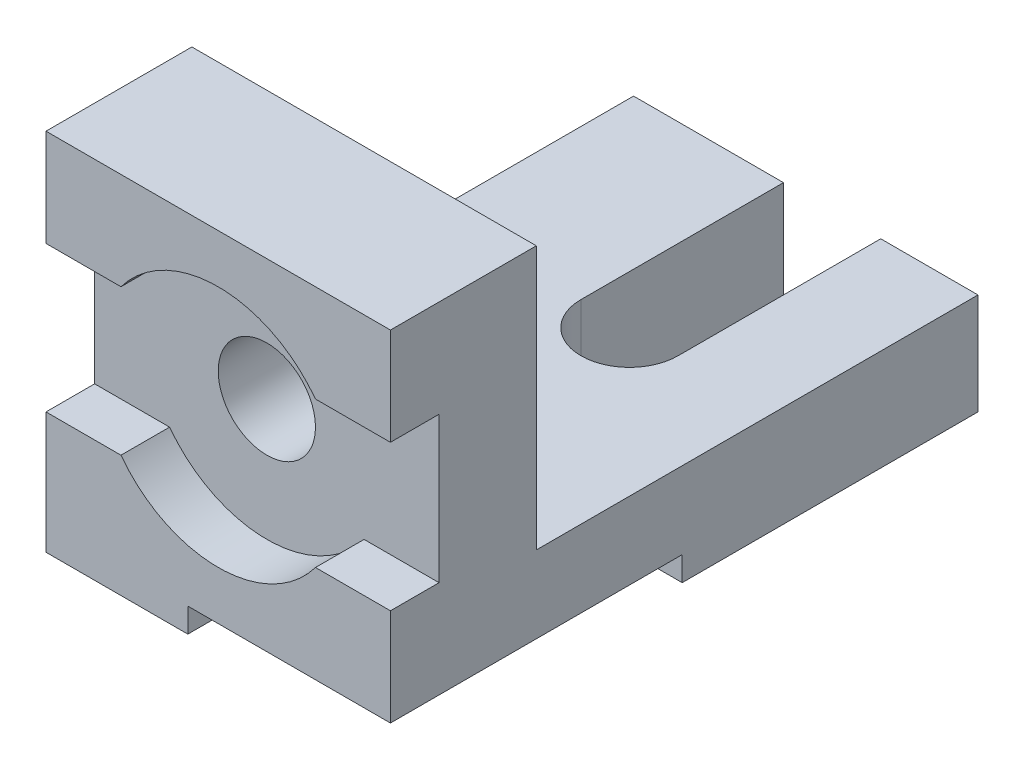
ISO-10303-21;
HEADER;
FILE_DESCRIPTION(('STEP AP214'),'2;1');
FILE_NAME('part.step','',(''),(''),'','','');
FILE_SCHEMA(('AUTOMOTIVE_DESIGN { 1 0 10303 214 1 1 1 1 }'));
ENDSEC;
DATA;
#1=APPLICATION_CONTEXT('core data for automotive mechanical design processes');
#2=APPLICATION_PROTOCOL_DEFINITION('international standard','automotive_design',2000,#1);
#3=PRODUCT_CONTEXT('',#1,'mechanical');
#4=PRODUCT('Part','Part','',(#3));
#5=PRODUCT_RELATED_PRODUCT_CATEGORY('part','',(#4));
#6=PRODUCT_DEFINITION_FORMATION('','',#4);
#7=PRODUCT_DEFINITION_CONTEXT('part definition',#1,'design');
#8=PRODUCT_DEFINITION('design','',#6,#7);
#9=PRODUCT_DEFINITION_SHAPE('','',#8);
#10=(LENGTH_UNIT() NAMED_UNIT(*) SI_UNIT(.MILLI.,.METRE.));
#11=(NAMED_UNIT(*) PLANE_ANGLE_UNIT() SI_UNIT($,.RADIAN.));
#12=(NAMED_UNIT(*) SI_UNIT($,.STERADIAN.) SOLID_ANGLE_UNIT());
#13=UNCERTAINTY_MEASURE_WITH_UNIT(LENGTH_MEASURE(1.E-05),#10,'distance_accuracy_value','');
#14=(GEOMETRIC_REPRESENTATION_CONTEXT(3) GLOBAL_UNCERTAINTY_ASSIGNED_CONTEXT((#13)) GLOBAL_UNIT_ASSIGNED_CONTEXT((#10,
#11,#12)) REPRESENTATION_CONTEXT('',''));
#15=CARTESIAN_POINT('',(0.,0.,0.));
#16=DIRECTION('',(0.,0.,1.));
#17=DIRECTION('',(1.,0.,0.));
#18=AXIS2_PLACEMENT_3D('',#15,#16,#17);
#19=CARTESIAN_POINT('',(42.5,0.,95.));
#20=DIRECTION('',(0.,0.,-1.));
#21=DIRECTION('',(-1.,0.,0.));
#22=AXIS2_PLACEMENT_3D('',#19,#20,#21);
#23=PLANE('',#22);
#24=DIRECTION('',(1.,0.,0.));
#25=VECTOR('',#24,1.);
#26=CARTESIAN_POINT('',(0.,30.,95.));
#27=LINE('',#26,#25);
#28=CARTESIAN_POINT('',(-42.5,30.,95.));
#29=VERTEX_POINT('',#28);
#30=CARTESIAN_POINT('',(-24.,30.,95.));
#31=VERTEX_POINT('',#30);
#32=EDGE_CURVE('E229',#29,#31,#27,.T.);
#33=ORIENTED_EDGE('',*,*,#32,.F.);
#34=DIRECTION('',(0.,-1.,0.));
#35=VECTOR('',#34,1.);
#36=CARTESIAN_POINT('',(-42.5,0.,95.));
#37=LINE('',#36,#35);
#38=CARTESIAN_POINT('',(-42.5,0.,95.));
#39=VERTEX_POINT('',#38);
#40=EDGE_CURVE('E314',#29,#39,#37,.T.);
#41=ORIENTED_EDGE('',*,*,#40,.T.);
#42=DIRECTION('',(-1.,0.,0.));
#43=VECTOR('',#42,1.);
#44=CARTESIAN_POINT('',(42.5,0.,95.));
#45=LINE('',#44,#43);
#46=CARTESIAN_POINT('',(-7.5,0.,95.));
#47=VERTEX_POINT('',#46);
#48=EDGE_CURVE('E323',#47,#39,#45,.T.);
#49=ORIENTED_EDGE('',*,*,#48,.F.);
#50=DIRECTION('',(0.,-1.,0.));
#51=VECTOR('',#50,1.);
#52=CARTESIAN_POINT('',(-7.5,0.,95.));
#53=LINE('',#52,#51);
#54=CARTESIAN_POINT('',(-7.5,5.99999999999996,95.));
#55=VERTEX_POINT('',#54);
#56=EDGE_CURVE('E258',#55,#47,#53,.T.);
#57=ORIENTED_EDGE('',*,*,#56,.F.);
#58=DIRECTION('',(1.,0.,0.));
#59=VECTOR('',#58,1.);
#60=CARTESIAN_POINT('',(-7.5,5.99999999999996,95.));
#61=LINE('',#60,#59);
#62=CARTESIAN_POINT('',(42.5,5.99999999999996,95.));
#63=VERTEX_POINT('',#62);
#64=EDGE_CURVE('E268',#55,#63,#61,.T.);
#65=ORIENTED_EDGE('',*,*,#64,.T.);
#66=DIRECTION('',(0.,-1.,0.));
#67=VECTOR('',#66,1.);
#68=CARTESIAN_POINT('',(42.5,0.,95.));
#69=LINE('',#68,#67);
#70=CARTESIAN_POINT('',(42.5,30.,95.));
#71=VERTEX_POINT('',#70);
#72=EDGE_CURVE('E300',#71,#63,#69,.T.);
#73=ORIENTED_EDGE('',*,*,#72,.F.);
#74=DIRECTION('',(1.,0.,0.));
#75=VECTOR('',#74,1.);
#76=CARTESIAN_POINT('',(0.,30.,95.));
#77=LINE('',#76,#75);
#78=CARTESIAN_POINT('',(24.,30.,95.));
#79=VERTEX_POINT('',#78);
#80=EDGE_CURVE('E203',#79,#71,#77,.T.);
#81=ORIENTED_EDGE('',*,*,#80,.F.);
#82=CARTESIAN_POINT('',(0.,48.,95.));
#83=DIRECTION('',(0.,0.,1.));
#84=DIRECTION('',(1.,0.,0.));
#85=AXIS2_PLACEMENT_3D('',#82,#83,#84);
#86=CIRCLE('',#85,30.);
#87=EDGE_CURVE('E226',#31,#79,#86,.T.);
#88=ORIENTED_EDGE('',*,*,#87,.F.);
#89=EDGE_LOOP('',(#33,#41,#49,#57,#65,#73,#81,#88));
#90=FACE_BOUND('',#89,.T.);
#91=ADVANCED_FACE('F39',(#90),#23,.F.);
#92=CARTESIAN_POINT('',(-42.5,0.,0.));
#93=DIRECTION('',(-1.,0.,0.));
#94=DIRECTION('',(0.,0.,1.));
#95=AXIS2_PLACEMENT_3D('',#92,#93,#94);
#96=PLANE('',#95);
#97=DIRECTION('',(0.,-1.,0.));
#98=VECTOR('',#97,1.);
#99=CARTESIAN_POINT('',(-42.5,0.,83.));
#100=LINE('',#99,#98);
#101=CARTESIAN_POINT('',(-42.5,66.,83.));
#102=VERTEX_POINT('',#101);
#103=CARTESIAN_POINT('',(-42.5,30.,83.));
#104=VERTEX_POINT('',#103);
#105=EDGE_CURVE('E206',#102,#104,#100,.T.);
#106=ORIENTED_EDGE('',*,*,#105,.F.);
#107=DIRECTION('',(0.,0.,1.));
#108=VECTOR('',#107,1.);
#109=CARTESIAN_POINT('',(-42.5,66.,83.));
#110=LINE('',#109,#108);
#111=CARTESIAN_POINT('',(-42.5,66.,95.));
#112=VERTEX_POINT('',#111);
#113=EDGE_CURVE('E241',#102,#112,#110,.T.);
#114=ORIENTED_EDGE('',*,*,#113,.T.);
#115=CARTESIAN_POINT('',(-42.5,90.,95.));
#116=VERTEX_POINT('',#115);
#117=EDGE_CURVE('E312',#116,#112,#37,.T.);
#118=ORIENTED_EDGE('',*,*,#117,.F.);
#119=DIRECTION('',(0.,0.,1.));
#120=VECTOR('',#119,1.);
#121=CARTESIAN_POINT('',(-42.5,90.,95.));
#122=LINE('',#121,#120);
#123=CARTESIAN_POINT('',(-42.5,90.,59.));
#124=VERTEX_POINT('',#123);
#125=EDGE_CURVE('E315',#124,#116,#122,.T.);
#126=ORIENTED_EDGE('',*,*,#125,.F.);
#127=DIRECTION('',(0.,1.,0.));
#128=VECTOR('',#127,1.);
#129=CARTESIAN_POINT('',(-42.5,90.,59.));
#130=LINE('',#129,#128);
#131=CARTESIAN_POINT('',(-42.5,25.,59.));
#132=VERTEX_POINT('',#131);
#133=EDGE_CURVE('E309',#132,#124,#130,.T.);
#134=ORIENTED_EDGE('',*,*,#133,.F.);
#135=DIRECTION('',(0.,0.,1.));
#136=VECTOR('',#135,1.);
#137=CARTESIAN_POINT('',(-42.5,25.,59.));
#138=LINE('',#137,#136);
#139=CARTESIAN_POINT('',(-42.5,25.,-50.));
#140=VERTEX_POINT('',#139);
#141=EDGE_CURVE('E306',#140,#132,#138,.T.);
#142=ORIENTED_EDGE('',*,*,#141,.F.);
#143=DIRECTION('',(0.,1.,0.));
#144=VECTOR('',#143,1.);
#145=CARTESIAN_POINT('',(-42.5,25.,-50.));
#146=LINE('',#145,#144);
#147=CARTESIAN_POINT('',(-42.5,0.,-50.));
#148=VERTEX_POINT('',#147);
#149=EDGE_CURVE('E284',#148,#140,#146,.T.);
#150=ORIENTED_EDGE('',*,*,#149,.F.);
#151=DIRECTION('',(0.,0.,-1.));
#152=VECTOR('',#151,1.);
#153=CARTESIAN_POINT('',(-42.5,0.,-50.));
#154=LINE('',#153,#152);
#155=EDGE_CURVE('E291',#39,#148,#154,.T.);
#156=ORIENTED_EDGE('',*,*,#155,.F.);
#157=ORIENTED_EDGE('',*,*,#40,.F.);
#158=DIRECTION('',(0.,0.,1.));
#159=VECTOR('',#158,1.);
#160=CARTESIAN_POINT('',(-42.5,30.,83.));
#161=LINE('',#160,#159);
#162=EDGE_CURVE('E242',#104,#29,#161,.T.);
#163=ORIENTED_EDGE('',*,*,#162,.F.);
#164=EDGE_LOOP('',(#106,#114,#118,#126,#134,#142,#150,#156,#157,#163));
#165=FACE_BOUND('',#164,.T.);
#166=ADVANCED_FACE('F387',(#165),#96,.T.);
#167=CARTESIAN_POINT('',(42.5,0.,-50.));
#168=DIRECTION('',(0.,1.,0.));
#169=DIRECTION('',(0.,0.,1.));
#170=AXIS2_PLACEMENT_3D('',#167,#168,#169);
#171=PLANE('',#170);
#172=DIRECTION('',(0.,0.,-1.));
#173=VECTOR('',#172,1.);
#174=CARTESIAN_POINT('',(-7.5,0.,23.));
#175=LINE('',#174,#173);
#176=CARTESIAN_POINT('',(-7.5,0.,23.));
#177=VERTEX_POINT('',#176);
#178=EDGE_CURVE('E256',#47,#177,#175,.T.);
#179=ORIENTED_EDGE('',*,*,#178,.F.);
#180=ORIENTED_EDGE('',*,*,#48,.T.);
#181=ORIENTED_EDGE('',*,*,#155,.T.);
#182=DIRECTION('',(-1.,0.,0.));
#183=VECTOR('',#182,1.);
#184=CARTESIAN_POINT('',(42.5,0.,-50.));
#185=LINE('',#184,#183);
#186=CARTESIAN_POINT('',(-5.5,0.,-50.));
#187=VERTEX_POINT('',#186);
#188=EDGE_CURVE('E304',#187,#148,#185,.T.);
#189=ORIENTED_EDGE('',*,*,#188,.F.);
#190=DIRECTION('',(0.,0.,1.));
#191=VECTOR('',#190,1.);
#192=CARTESIAN_POINT('',(-5.5,0.,-50.));
#193=LINE('',#192,#191);
#194=CARTESIAN_POINT('',(-5.5,0.,0.));
#195=VERTEX_POINT('',#194);
#196=EDGE_CURVE('E11',#187,#195,#193,.T.);
#197=ORIENTED_EDGE('',*,*,#196,.T.);
#198=CARTESIAN_POINT('',(6.5,0.,0.));
#199=DIRECTION('',(0.,1.,0.));
#200=DIRECTION('',(0.,0.,1.));
#201=AXIS2_PLACEMENT_3D('',#198,#199,#200);
#202=CIRCLE('',#201,12.);
#203=CARTESIAN_POINT('',(18.5,0.,0.));
#204=VERTEX_POINT('',#203);
#205=EDGE_CURVE('E50',#195,#204,#202,.T.);
#206=ORIENTED_EDGE('',*,*,#205,.T.);
#207=DIRECTION('',(0.,0.,-1.));
#208=VECTOR('',#207,1.);
#209=CARTESIAN_POINT('',(18.5,0.,-50.));
#210=LINE('',#209,#208);
#211=CARTESIAN_POINT('',(18.5,0.,-50.));
#212=VERTEX_POINT('',#211);
#213=EDGE_CURVE('E340',#204,#212,#210,.T.);
#214=ORIENTED_EDGE('',*,*,#213,.T.);
#215=CARTESIAN_POINT('',(42.5,0.,-50.));
#216=VERTEX_POINT('',#215);
#217=EDGE_CURVE('E319',#216,#212,#185,.T.);
#218=ORIENTED_EDGE('',*,*,#217,.F.);
#219=DIRECTION('',(0.,0.,-1.));
#220=VECTOR('',#219,1.);
#221=CARTESIAN_POINT('',(42.5,0.,-50.));
#222=LINE('',#221,#220);
#223=CARTESIAN_POINT('',(42.5,0.,23.));
#224=VERTEX_POINT('',#223);
#225=EDGE_CURVE('E302',#224,#216,#222,.T.);
#226=ORIENTED_EDGE('',*,*,#225,.F.);
#227=DIRECTION('',(1.,0.,0.));
#228=VECTOR('',#227,1.);
#229=CARTESIAN_POINT('',(-7.5,0.,23.));
#230=LINE('',#229,#228);
#231=EDGE_CURVE('E264',#177,#224,#230,.T.);
#232=ORIENTED_EDGE('',*,*,#231,.F.);
#233=EDGE_LOOP('',(#179,#180,#181,#189,#197,#206,#214,#218,#226,#232));
#234=FACE_BOUND('',#233,.T.);
#235=ADVANCED_FACE('F343',(#234),#171,.F.);
#236=CARTESIAN_POINT('',(42.5,0.,0.));
#237=DIRECTION('',(-1.,0.,0.));
#238=DIRECTION('',(0.,0.,1.));
#239=AXIS2_PLACEMENT_3D('',#236,#237,#238);
#240=PLANE('',#239);
#241=DIRECTION('',(0.,1.,0.));
#242=VECTOR('',#241,1.);
#243=CARTESIAN_POINT('',(42.5,0.,83.));
#244=LINE('',#243,#242);
#245=CARTESIAN_POINT('',(42.5,30.,83.));
#246=VERTEX_POINT('',#245);
#247=CARTESIAN_POINT('',(42.5,66.,83.));
#248=VERTEX_POINT('',#247);
#249=EDGE_CURVE('E193',#246,#248,#244,.T.);
#250=ORIENTED_EDGE('',*,*,#249,.F.);
#251=DIRECTION('',(0.,0.,1.));
#252=VECTOR('',#251,1.);
#253=CARTESIAN_POINT('',(42.5,30.,83.));
#254=LINE('',#253,#252);
#255=EDGE_CURVE('E237',#246,#71,#254,.T.);
#256=ORIENTED_EDGE('',*,*,#255,.T.);
#257=ORIENTED_EDGE('',*,*,#72,.T.);
#258=DIRECTION('',(0.,0.,1.));
#259=VECTOR('',#258,1.);
#260=CARTESIAN_POINT('',(42.5,5.99999999999998,23.));
#261=LINE('',#260,#259);
#262=CARTESIAN_POINT('',(42.5,5.99999999999998,23.));
#263=VERTEX_POINT('',#262);
#264=EDGE_CURVE('E251',#263,#63,#261,.T.);
#265=ORIENTED_EDGE('',*,*,#264,.F.);
#266=DIRECTION('',(0.,1.,0.));
#267=VECTOR('',#266,1.);
#268=CARTESIAN_POINT('',(42.5,0.,23.));
#269=LINE('',#268,#267);
#270=EDGE_CURVE('E64',#224,#263,#269,.T.);
#271=ORIENTED_EDGE('',*,*,#270,.F.);
#272=ORIENTED_EDGE('',*,*,#225,.T.);
#273=DIRECTION('',(0.,1.,0.));
#274=VECTOR('',#273,1.);
#275=CARTESIAN_POINT('',(42.5,25.,-50.));
#276=LINE('',#275,#274);
#277=CARTESIAN_POINT('',(42.5,25.,-50.));
#278=VERTEX_POINT('',#277);
#279=EDGE_CURVE('E288',#216,#278,#276,.T.);
#280=ORIENTED_EDGE('',*,*,#279,.T.);
#281=DIRECTION('',(0.,0.,1.));
#282=VECTOR('',#281,1.);
#283=CARTESIAN_POINT('',(42.5,25.,59.));
#284=LINE('',#283,#282);
#285=CARTESIAN_POINT('',(42.5,25.,59.));
#286=VERTEX_POINT('',#285);
#287=EDGE_CURVE('E295',#278,#286,#284,.T.);
#288=ORIENTED_EDGE('',*,*,#287,.T.);
#289=DIRECTION('',(0.,1.,0.));
#290=VECTOR('',#289,1.);
#291=CARTESIAN_POINT('',(42.5,90.,59.));
#292=LINE('',#291,#290);
#293=CARTESIAN_POINT('',(42.5,90.,59.));
#294=VERTEX_POINT('',#293);
#295=EDGE_CURVE('E293',#286,#294,#292,.T.);
#296=ORIENTED_EDGE('',*,*,#295,.T.);
#297=DIRECTION('',(0.,0.,1.));
#298=VECTOR('',#297,1.);
#299=CARTESIAN_POINT('',(42.5,90.,95.));
#300=LINE('',#299,#298);
#301=CARTESIAN_POINT('',(42.5,90.,95.));
#302=VERTEX_POINT('',#301);
#303=EDGE_CURVE('E299',#294,#302,#300,.T.);
#304=ORIENTED_EDGE('',*,*,#303,.T.);
#305=CARTESIAN_POINT('',(42.5,66.,95.));
#306=VERTEX_POINT('',#305);
#307=EDGE_CURVE('E296',#302,#306,#69,.T.);
#308=ORIENTED_EDGE('',*,*,#307,.T.);
#309=DIRECTION('',(0.,0.,1.));
#310=VECTOR('',#309,1.);
#311=CARTESIAN_POINT('',(42.5,66.,83.));
#312=LINE('',#311,#310);
#313=EDGE_CURVE('E233',#248,#306,#312,.T.);
#314=ORIENTED_EDGE('',*,*,#313,.F.);
#315=EDGE_LOOP('',(#250,#256,#257,#265,#271,#272,#280,#288,#296,#304,#308,#314));
#316=FACE_BOUND('',#315,.T.);
#317=ADVANCED_FACE('F366',(#316),#240,.F.);
#318=CARTESIAN_POINT('',(42.5,25.,-50.));
#319=DIRECTION('',(0.,0.,1.));
#320=DIRECTION('',(1.,0.,0.));
#321=AXIS2_PLACEMENT_3D('',#318,#319,#320);
#322=PLANE('',#321);
#323=DIRECTION('',(0.,1.,0.));
#324=VECTOR('',#323,1.);
#325=CARTESIAN_POINT('',(-5.5,-60.,-50.));
#326=LINE('',#325,#324);
#327=CARTESIAN_POINT('',(-5.5,25.,-50.));
#328=VERTEX_POINT('',#327);
#329=EDGE_CURVE('E282',#187,#328,#326,.T.);
#330=ORIENTED_EDGE('',*,*,#329,.F.);
#331=ORIENTED_EDGE('',*,*,#188,.T.);
#332=ORIENTED_EDGE('',*,*,#149,.T.);
#333=DIRECTION('',(-1.,0.,0.));
#334=VECTOR('',#333,1.);
#335=CARTESIAN_POINT('',(42.5,25.,-50.));
#336=LINE('',#335,#334);
#337=EDGE_CURVE('E333',#328,#140,#336,.T.);
#338=ORIENTED_EDGE('',*,*,#337,.F.);
#339=EDGE_LOOP('',(#330,#331,#332,#338));
#340=FACE_BOUND('',#339,.T.);
#341=ADVANCED_FACE('F393',(#340),#322,.F.);
#342=CARTESIAN_POINT('',(42.5,25.,59.));
#343=DIRECTION('',(0.,-1.,0.));
#344=DIRECTION('',(0.,0.,-1.));
#345=AXIS2_PLACEMENT_3D('',#342,#343,#344);
#346=PLANE('',#345);
#347=DIRECTION('',(0.,0.,-1.));
#348=VECTOR('',#347,1.);
#349=CARTESIAN_POINT('',(18.5,25.,0.));
#350=LINE('',#349,#348);
#351=CARTESIAN_POINT('',(18.5,25.,0.));
#352=VERTEX_POINT('',#351);
#353=CARTESIAN_POINT('',(18.5,25.,-50.));
#354=VERTEX_POINT('',#353);
#355=EDGE_CURVE('E273',#352,#354,#350,.T.);
#356=ORIENTED_EDGE('',*,*,#355,.F.);
#357=CARTESIAN_POINT('',(6.5,25.,0.));
#358=DIRECTION('',(0.,1.,0.));
#359=DIRECTION('',(0.,0.,1.));
#360=AXIS2_PLACEMENT_3D('',#357,#358,#359);
#361=CIRCLE('',#360,12.);
#362=CARTESIAN_POINT('',(-5.5,25.,0.));
#363=VERTEX_POINT('',#362);
#364=EDGE_CURVE('E270',#363,#352,#361,.T.);
#365=ORIENTED_EDGE('',*,*,#364,.F.);
#366=DIRECTION('',(0.,0.,1.));
#367=VECTOR('',#366,1.);
#368=CARTESIAN_POINT('',(-5.5,25.,0.));
#369=LINE('',#368,#367);
#370=EDGE_CURVE('E277',#328,#363,#369,.T.);
#371=ORIENTED_EDGE('',*,*,#370,.F.);
#372=ORIENTED_EDGE('',*,*,#337,.T.);
#373=ORIENTED_EDGE('',*,*,#141,.T.);
#374=DIRECTION('',(-1.,0.,0.));
#375=VECTOR('',#374,1.);
#376=CARTESIAN_POINT('',(42.5,25.,59.));
#377=LINE('',#376,#375);
#378=EDGE_CURVE('E335',#286,#132,#377,.T.);
#379=ORIENTED_EDGE('',*,*,#378,.F.);
#380=ORIENTED_EDGE('',*,*,#287,.F.);
#381=EDGE_CURVE('E338',#278,#354,#336,.T.);
#382=ORIENTED_EDGE('',*,*,#381,.T.);
#383=EDGE_LOOP('',(#356,#365,#371,#372,#373,#379,#380,#382));
#384=FACE_BOUND('',#383,.T.);
#385=ADVANCED_FACE('F358',(#384),#346,.F.);
#386=ORIENTED_EDGE('',*,*,#217,.T.);
#387=DIRECTION('',(0.,1.,0.));
#388=VECTOR('',#387,1.);
#389=CARTESIAN_POINT('',(18.5,-60.,-50.));
#390=LINE('',#389,#388);
#391=EDGE_CURVE('E281',#212,#354,#390,.T.);
#392=ORIENTED_EDGE('',*,*,#391,.T.);
#393=ORIENTED_EDGE('',*,*,#381,.F.);
#394=ORIENTED_EDGE('',*,*,#279,.F.);
#395=EDGE_LOOP('',(#386,#392,#393,#394));
#396=FACE_BOUND('',#395,.T.);
#397=ADVANCED_FACE('F41',(#396),#322,.F.);
#398=CARTESIAN_POINT('',(42.5,90.,59.));
#399=DIRECTION('',(0.,0.,1.));
#400=DIRECTION('',(0.,-1.,0.));
#401=AXIS2_PLACEMENT_3D('',#398,#399,#400);
#402=PLANE('',#401);
#403=CARTESIAN_POINT('',(0.,48.,59.));
#404=DIRECTION('',(0.,0.,1.));
#405=DIRECTION('',(0.,-1.,0.));
#406=AXIS2_PLACEMENT_3D('',#403,#404,#405);
#407=CIRCLE('',#406,12.);
#408=CARTESIAN_POINT('',(0.,36.,59.));
#409=VERTEX_POINT('',#408);
#410=EDGE_CURVE('E225',#409,#409,#407,.F.);
#411=ORIENTED_EDGE('',*,*,#410,.F.);
#412=EDGE_LOOP('',(#411));
#413=FACE_BOUND('',#412,.T.);
#414=ORIENTED_EDGE('',*,*,#133,.T.);
#415=DIRECTION('',(-1.,0.,0.));
#416=VECTOR('',#415,1.);
#417=CARTESIAN_POINT('',(42.5,90.,59.));
#418=LINE('',#417,#416);
#419=EDGE_CURVE('E328',#294,#124,#418,.T.);
#420=ORIENTED_EDGE('',*,*,#419,.F.);
#421=ORIENTED_EDGE('',*,*,#295,.F.);
#422=ORIENTED_EDGE('',*,*,#378,.T.);
#423=EDGE_LOOP('',(#414,#420,#421,#422));
#424=FACE_BOUND('',#423,.T.);
#425=ADVANCED_FACE('F391',(#413,#424),#402,.F.);
#426=CARTESIAN_POINT('',(42.5,90.,95.));
#427=DIRECTION('',(0.,-1.,0.));
#428=DIRECTION('',(0.,0.,-1.));
#429=AXIS2_PLACEMENT_3D('',#426,#427,#428);
#430=PLANE('',#429);
#431=ORIENTED_EDGE('',*,*,#125,.T.);
#432=DIRECTION('',(-1.,0.,0.));
#433=VECTOR('',#432,1.);
#434=CARTESIAN_POINT('',(42.5,90.,95.));
#435=LINE('',#434,#433);
#436=EDGE_CURVE('E326',#302,#116,#435,.T.);
#437=ORIENTED_EDGE('',*,*,#436,.F.);
#438=ORIENTED_EDGE('',*,*,#303,.F.);
#439=ORIENTED_EDGE('',*,*,#419,.T.);
#440=EDGE_LOOP('',(#431,#437,#438,#439));
#441=FACE_BOUND('',#440,.T.);
#442=ADVANCED_FACE('F402',(#441),#430,.F.);
#443=CARTESIAN_POINT('',(0.,48.,95.));
#444=DIRECTION('',(0.,0.,1.));
#445=DIRECTION('',(1.,0.,0.));
#446=AXIS2_PLACEMENT_3D('',#443,#444,#445);
#447=CIRCLE('',#446,30.);
#448=CARTESIAN_POINT('',(24.,66.,95.));
#449=VERTEX_POINT('',#448);
#450=CARTESIAN_POINT('',(-24.,66.,95.));
#451=VERTEX_POINT('',#450);
#452=EDGE_CURVE('E222',#449,#451,#447,.T.);
#453=ORIENTED_EDGE('',*,*,#452,.F.);
#454=DIRECTION('',(1.,0.,0.));
#455=VECTOR('',#454,1.);
#456=CARTESIAN_POINT('',(0.,66.,95.));
#457=LINE('',#456,#455);
#458=EDGE_CURVE('E187',#449,#306,#457,.T.);
#459=ORIENTED_EDGE('',*,*,#458,.T.);
#460=ORIENTED_EDGE('',*,*,#307,.F.);
#461=ORIENTED_EDGE('',*,*,#436,.T.);
#462=ORIENTED_EDGE('',*,*,#117,.T.);
#463=DIRECTION('',(1.,0.,0.));
#464=VECTOR('',#463,1.);
#465=CARTESIAN_POINT('',(0.,66.,95.));
#466=LINE('',#465,#464);
#467=EDGE_CURVE('E221',#112,#451,#466,.T.);
#468=ORIENTED_EDGE('',*,*,#467,.T.);
#469=EDGE_LOOP('',(#453,#459,#460,#461,#462,#468));
#470=FACE_BOUND('',#469,.T.);
#471=ADVANCED_FACE('F403',(#470),#23,.F.);
#472=CARTESIAN_POINT('',(6.5,-60.,0.));
#473=DIRECTION('',(0.,1.,0.));
#474=DIRECTION('',(0.,0.,1.));
#475=AXIS2_PLACEMENT_3D('',#472,#473,#474);
#476=CYLINDRICAL_SURFACE('',#475,12.);
#477=DIRECTION('',(0.,1.,0.));
#478=VECTOR('',#477,1.);
#479=CARTESIAN_POINT('',(-5.5,-60.,0.));
#480=LINE('',#479,#478);
#481=EDGE_CURVE('E278',#195,#363,#480,.T.);
#482=ORIENTED_EDGE('',*,*,#481,.T.);
#483=ORIENTED_EDGE('',*,*,#364,.T.);
#484=DIRECTION('',(0.,1.,0.));
#485=VECTOR('',#484,1.);
#486=CARTESIAN_POINT('',(18.5,-60.,0.));
#487=LINE('',#486,#485);
#488=EDGE_CURVE('E276',#204,#352,#487,.T.);
#489=ORIENTED_EDGE('',*,*,#488,.F.);
#490=ORIENTED_EDGE('',*,*,#205,.F.);
#491=EDGE_LOOP('',(#482,#483,#489,#490));
#492=FACE_BOUND('',#491,.T.);
#493=ADVANCED_FACE('F348',(#492),#476,.F.);
#494=CARTESIAN_POINT('',(-5.5,-60.,0.));
#495=DIRECTION('',(-1.,0.,0.));
#496=DIRECTION('',(0.,0.,1.));
#497=AXIS2_PLACEMENT_3D('',#494,#495,#496);
#498=PLANE('',#497);
#499=ORIENTED_EDGE('',*,*,#329,.T.);
#500=ORIENTED_EDGE('',*,*,#370,.T.);
#501=ORIENTED_EDGE('',*,*,#481,.F.);
#502=ORIENTED_EDGE('',*,*,#196,.F.);
#503=EDGE_LOOP('',(#499,#500,#501,#502));
#504=FACE_BOUND('',#503,.T.);
#505=ADVANCED_FACE('F354',(#504),#498,.F.);
#506=CARTESIAN_POINT('',(18.5,-60.,0.));
#507=DIRECTION('',(1.,0.,0.));
#508=DIRECTION('',(0.,0.,-1.));
#509=AXIS2_PLACEMENT_3D('',#506,#507,#508);
#510=PLANE('',#509);
#511=ORIENTED_EDGE('',*,*,#488,.T.);
#512=ORIENTED_EDGE('',*,*,#355,.T.);
#513=ORIENTED_EDGE('',*,*,#391,.F.);
#514=ORIENTED_EDGE('',*,*,#213,.F.);
#515=EDGE_LOOP('',(#511,#512,#513,#514));
#516=FACE_BOUND('',#515,.T.);
#517=ADVANCED_FACE('F362',(#516),#510,.F.);
#518=CARTESIAN_POINT('',(-7.5,0.,23.));
#519=DIRECTION('',(0.,0.,-1.));
#520=DIRECTION('',(-1.,0.,0.));
#521=AXIS2_PLACEMENT_3D('',#518,#519,#520);
#522=PLANE('',#521);
#523=ORIENTED_EDGE('',*,*,#270,.T.);
#524=DIRECTION('',(1.,0.,0.));
#525=VECTOR('',#524,1.);
#526=CARTESIAN_POINT('',(-7.5,5.99999999999998,23.));
#527=LINE('',#526,#525);
#528=CARTESIAN_POINT('',(-7.5,5.99999999999998,23.));
#529=VERTEX_POINT('',#528);
#530=EDGE_CURVE('E261',#529,#263,#527,.T.);
#531=ORIENTED_EDGE('',*,*,#530,.F.);
#532=DIRECTION('',(0.,1.,0.));
#533=VECTOR('',#532,1.);
#534=CARTESIAN_POINT('',(-7.5,0.,23.));
#535=LINE('',#534,#533);
#536=EDGE_CURVE('E248',#177,#529,#535,.T.);
#537=ORIENTED_EDGE('',*,*,#536,.F.);
#538=ORIENTED_EDGE('',*,*,#231,.T.);
#539=EDGE_LOOP('',(#523,#531,#537,#538));
#540=FACE_BOUND('',#539,.T.);
#541=ADVANCED_FACE('F463',(#540),#522,.F.);
#542=CARTESIAN_POINT('',(-7.5,5.99999999999998,23.));
#543=DIRECTION('',(0.,1.,0.));
#544=DIRECTION('',(0.,0.,1.));
#545=AXIS2_PLACEMENT_3D('',#542,#543,#544);
#546=PLANE('',#545);
#547=ORIENTED_EDGE('',*,*,#264,.T.);
#548=ORIENTED_EDGE('',*,*,#64,.F.);
#549=DIRECTION('',(0.,0.,1.));
#550=VECTOR('',#549,1.);
#551=CARTESIAN_POINT('',(-7.5,5.99999999999998,23.));
#552=LINE('',#551,#550);
#553=EDGE_CURVE('E252',#529,#55,#552,.T.);
#554=ORIENTED_EDGE('',*,*,#553,.F.);
#555=ORIENTED_EDGE('',*,*,#530,.T.);
#556=EDGE_LOOP('',(#547,#548,#554,#555));
#557=FACE_BOUND('',#556,.T.);
#558=ADVANCED_FACE('F375',(#557),#546,.F.);
#559=CARTESIAN_POINT('',(-7.5,0.,0.));
#560=DIRECTION('',(1.,0.,0.));
#561=DIRECTION('',(0.,0.,-1.));
#562=AXIS2_PLACEMENT_3D('',#559,#560,#561);
#563=PLANE('',#562);
#564=ORIENTED_EDGE('',*,*,#536,.T.);
#565=ORIENTED_EDGE('',*,*,#553,.T.);
#566=ORIENTED_EDGE('',*,*,#56,.T.);
#567=ORIENTED_EDGE('',*,*,#178,.T.);
#568=EDGE_LOOP('',(#564,#565,#566,#567));
#569=FACE_BOUND('',#568,.T.);
#570=ADVANCED_FACE('F379',(#569),#563,.T.);
#571=CARTESIAN_POINT('',(0.,66.,83.));
#572=DIRECTION('',(0.,-1.,0.));
#573=DIRECTION('',(0.,0.,-1.));
#574=AXIS2_PLACEMENT_3D('',#571,#572,#573);
#575=PLANE('',#574);
#576=ORIENTED_EDGE('',*,*,#458,.F.);
#577=DIRECTION('',(0.,0.,1.));
#578=VECTOR('',#577,1.);
#579=CARTESIAN_POINT('',(24.,66.,83.));
#580=LINE('',#579,#578);
#581=CARTESIAN_POINT('',(24.,66.,83.));
#582=VERTEX_POINT('',#581);
#583=EDGE_CURVE('E185',#582,#449,#580,.T.);
#584=ORIENTED_EDGE('',*,*,#583,.F.);
#585=DIRECTION('',(1.,0.,0.));
#586=VECTOR('',#585,1.);
#587=CARTESIAN_POINT('',(0.,66.,83.));
#588=LINE('',#587,#586);
#589=EDGE_CURVE('E183',#582,#248,#588,.T.);
#590=ORIENTED_EDGE('',*,*,#589,.T.);
#591=ORIENTED_EDGE('',*,*,#313,.T.);
#592=EDGE_LOOP('',(#576,#584,#590,#591));
#593=FACE_BOUND('',#592,.T.);
#594=ADVANCED_FACE('F184',(#593),#575,.T.);
#595=CARTESIAN_POINT('',(0.,30.,83.));
#596=DIRECTION('',(0.,-1.,0.));
#597=DIRECTION('',(0.,0.,-1.));
#598=AXIS2_PLACEMENT_3D('',#595,#596,#597);
#599=PLANE('',#598);
#600=ORIENTED_EDGE('',*,*,#80,.T.);
#601=ORIENTED_EDGE('',*,*,#255,.F.);
#602=DIRECTION('',(1.,0.,0.));
#603=VECTOR('',#602,1.);
#604=CARTESIAN_POINT('',(0.,30.,83.));
#605=LINE('',#604,#603);
#606=CARTESIAN_POINT('',(24.,30.,83.));
#607=VERTEX_POINT('',#606);
#608=EDGE_CURVE('E220',#607,#246,#605,.T.);
#609=ORIENTED_EDGE('',*,*,#608,.F.);
#610=DIRECTION('',(0.,0.,1.));
#611=VECTOR('',#610,1.);
#612=CARTESIAN_POINT('',(24.,30.,83.));
#613=LINE('',#612,#611);
#614=EDGE_CURVE('E239',#607,#79,#613,.T.);
#615=ORIENTED_EDGE('',*,*,#614,.T.);
#616=EDGE_LOOP('',(#600,#601,#609,#615));
#617=FACE_BOUND('',#616,.T.);
#618=ADVANCED_FACE('F407',(#617),#599,.F.);
#619=CARTESIAN_POINT('',(0.,48.,83.));
#620=DIRECTION('',(0.,0.,1.));
#621=DIRECTION('',(1.,0.,0.));
#622=AXIS2_PLACEMENT_3D('',#619,#620,#621);
#623=CYLINDRICAL_SURFACE('',#622,30.);
#624=ORIENTED_EDGE('',*,*,#87,.T.);
#625=ORIENTED_EDGE('',*,*,#614,.F.);
#626=CARTESIAN_POINT('',(0.,48.,83.));
#627=DIRECTION('',(0.,0.,1.));
#628=DIRECTION('',(1.,0.,0.));
#629=AXIS2_PLACEMENT_3D('',#626,#627,#628);
#630=CIRCLE('',#629,30.);
#631=CARTESIAN_POINT('',(-24.,30.,83.));
#632=VERTEX_POINT('',#631);
#633=EDGE_CURVE('E212',#632,#607,#630,.T.);
#634=ORIENTED_EDGE('',*,*,#633,.F.);
#635=DIRECTION('',(0.,0.,1.));
#636=VECTOR('',#635,1.);
#637=CARTESIAN_POINT('',(-24.,30.,83.));
#638=LINE('',#637,#636);
#639=EDGE_CURVE('E243',#632,#31,#638,.T.);
#640=ORIENTED_EDGE('',*,*,#639,.T.);
#641=EDGE_LOOP('',(#624,#625,#634,#640));
#642=FACE_BOUND('',#641,.T.);
#643=ADVANCED_FACE('F411',(#642),#623,.F.);
#644=CARTESIAN_POINT('',(0.,30.,83.));
#645=DIRECTION('',(0.,-1.,0.));
#646=DIRECTION('',(0.,0.,-1.));
#647=AXIS2_PLACEMENT_3D('',#644,#645,#646);
#648=PLANE('',#647);
#649=ORIENTED_EDGE('',*,*,#32,.T.);
#650=ORIENTED_EDGE('',*,*,#639,.F.);
#651=DIRECTION('',(1.,0.,0.));
#652=VECTOR('',#651,1.);
#653=CARTESIAN_POINT('',(0.,30.,83.));
#654=LINE('',#653,#652);
#655=EDGE_CURVE('E211',#104,#632,#654,.T.);
#656=ORIENTED_EDGE('',*,*,#655,.F.);
#657=ORIENTED_EDGE('',*,*,#162,.T.);
#658=EDGE_LOOP('',(#649,#650,#656,#657));
#659=FACE_BOUND('',#658,.T.);
#660=ADVANCED_FACE('F413',(#659),#648,.F.);
#661=CARTESIAN_POINT('',(0.,66.,83.));
#662=DIRECTION('',(0.,-1.,0.));
#663=DIRECTION('',(0.,0.,-1.));
#664=AXIS2_PLACEMENT_3D('',#661,#662,#663);
#665=PLANE('',#664);
#666=ORIENTED_EDGE('',*,*,#467,.F.);
#667=ORIENTED_EDGE('',*,*,#113,.F.);
#668=DIRECTION('',(1.,0.,0.));
#669=VECTOR('',#668,1.);
#670=CARTESIAN_POINT('',(0.,66.,83.));
#671=LINE('',#670,#669);
#672=CARTESIAN_POINT('',(-24.,66.,83.));
#673=VERTEX_POINT('',#672);
#674=EDGE_CURVE('E53',#102,#673,#671,.T.);
#675=ORIENTED_EDGE('',*,*,#674,.T.);
#676=DIRECTION('',(0.,0.,1.));
#677=VECTOR('',#676,1.);
#678=CARTESIAN_POINT('',(-24.,66.,83.));
#679=LINE('',#678,#677);
#680=EDGE_CURVE('E192',#673,#451,#679,.T.);
#681=ORIENTED_EDGE('',*,*,#680,.T.);
#682=EDGE_LOOP('',(#666,#667,#675,#681));
#683=FACE_BOUND('',#682,.T.);
#684=ADVANCED_FACE('F418',(#683),#665,.T.);
#685=CARTESIAN_POINT('',(0.,48.,83.));
#686=DIRECTION('',(0.,0.,1.));
#687=DIRECTION('',(1.,0.,0.));
#688=AXIS2_PLACEMENT_3D('',#685,#686,#687);
#689=CYLINDRICAL_SURFACE('',#688,30.);
#690=ORIENTED_EDGE('',*,*,#452,.T.);
#691=ORIENTED_EDGE('',*,*,#680,.F.);
#692=CARTESIAN_POINT('',(0.,48.,83.));
#693=DIRECTION('',(0.,0.,1.));
#694=DIRECTION('',(1.,0.,0.));
#695=AXIS2_PLACEMENT_3D('',#692,#693,#694);
#696=CIRCLE('',#695,30.);
#697=EDGE_CURVE('E197',#582,#673,#696,.T.);
#698=ORIENTED_EDGE('',*,*,#697,.F.);
#699=ORIENTED_EDGE('',*,*,#583,.T.);
#700=EDGE_LOOP('',(#690,#691,#698,#699));
#701=FACE_BOUND('',#700,.T.);
#702=ADVANCED_FACE('F204',(#701),#689,.F.);
#703=CARTESIAN_POINT('',(0.,0.,83.));
#704=DIRECTION('',(0.,0.,1.));
#705=DIRECTION('',(1.,0.,0.));
#706=AXIS2_PLACEMENT_3D('',#703,#704,#705);
#707=PLANE('',#706);
#708=CARTESIAN_POINT('',(0.,48.,83.));
#709=DIRECTION('',(0.,0.,1.));
#710=DIRECTION('',(1.,0.,0.));
#711=AXIS2_PLACEMENT_3D('',#708,#709,#710);
#712=CIRCLE('',#711,12.);
#713=CARTESIAN_POINT('',(12.,48.,83.));
#714=VERTEX_POINT('',#713);
#715=EDGE_CURVE('E487',#714,#714,#712,.F.);
#716=ORIENTED_EDGE('',*,*,#715,.T.);
#717=EDGE_LOOP('',(#716));
#718=FACE_BOUND('',#717,.T.);
#719=ORIENTED_EDGE('',*,*,#589,.F.);
#720=ORIENTED_EDGE('',*,*,#697,.T.);
#721=ORIENTED_EDGE('',*,*,#674,.F.);
#722=ORIENTED_EDGE('',*,*,#105,.T.);
#723=ORIENTED_EDGE('',*,*,#655,.T.);
#724=ORIENTED_EDGE('',*,*,#633,.T.);
#725=ORIENTED_EDGE('',*,*,#608,.T.);
#726=ORIENTED_EDGE('',*,*,#249,.T.);
#727=EDGE_LOOP('',(#719,#720,#721,#722,#723,#724,#725,#726));
#728=FACE_BOUND('',#727,.T.);
#729=ADVANCED_FACE('F198',(#718,#728),#707,.T.);
#730=CARTESIAN_POINT('',(0.,48.,-50.001));
#731=DIRECTION('',(0.,0.,1.));
#732=DIRECTION('',(1.,0.,0.));
#733=AXIS2_PLACEMENT_3D('',#730,#731,#732);
#734=CYLINDRICAL_SURFACE('',#733,12.);
#735=ORIENTED_EDGE('',*,*,#715,.F.);
#736=EDGE_LOOP('',(#735));
#737=FACE_BOUND('',#736,.T.);
#738=ORIENTED_EDGE('',*,*,#410,.T.);
#739=EDGE_LOOP('',(#738));
#740=FACE_BOUND('',#739,.T.);
#741=ADVANCED_FACE('F477',(#737,#740),#734,.F.);
#742=CLOSED_SHELL('',(#91,#166,#235,#317,#341,#385,#397,#425,#442,#471,#493,#505,#517,#541,#558,
#570,#594,#618,#643,#660,#684,#702,#729,#741));
#743=MANIFOLD_SOLID_BREP('B2',#742);
#744=ADVANCED_BREP_SHAPE_REPRESENTATION('',(#18,#743),#14);
#745=SHAPE_DEFINITION_REPRESENTATION(#9,#744);
ENDSEC;
END-ISO-10303-21;
